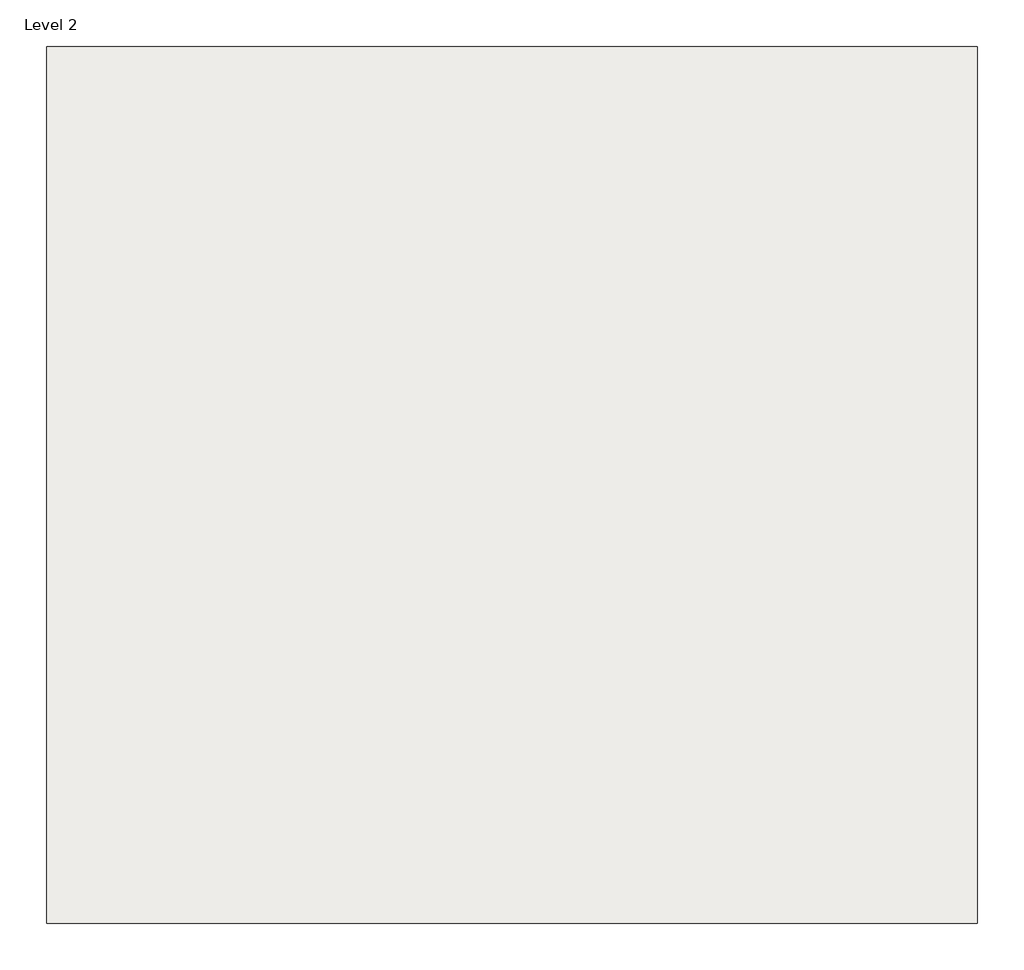
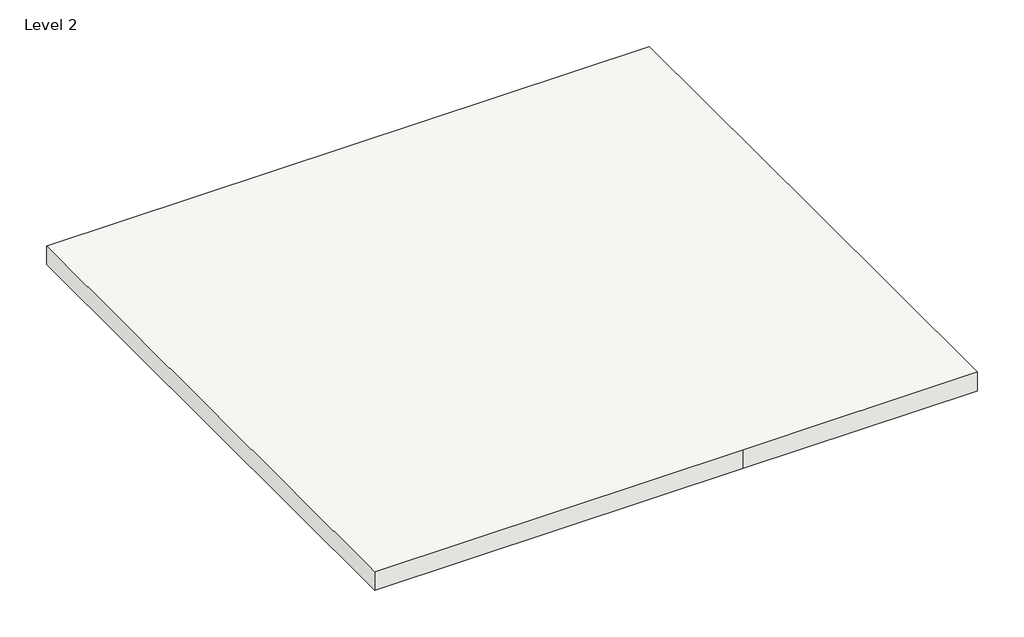
# One storey: 1 roof.
"""IFC4 building model written with IfcOpenShell, lengths in millimetres."""

from ifc_helpers import new_model, si_unit, frame, origin, place, context, project, spatial, polyline, outline, extrude, element, save

model = new_model("IFC4")

# Units and contexts
model_context = context("Model", 3, world=origin())
ifc_project = project(units=[si_unit("LENGTHUNIT", "METRE", prefix="MILLI")], contexts=[model_context])

# Site, building, storey
site = spatial("IfcSite", under=ifc_project)
building = spatial("IfcBuilding", under=site)
storey = spatial("IfcBuildingStorey", under=building, Name="Level 2", Elevation=3048.0)

# Roof
placement = place(None, origin())
element("IfcRoof", 1, ObjectType="Generic - 12\"", at=placement, inside=storey, context=model_context, shape_type="SweptSolid", body=[
    extrude(outline(polyline([(-13352.2770189, 15181.9523405), (-4081.2770189, 15181.9523405), (-4081.2770189, 10762.3523405), (-4081.2770189, 6444.3523405), (-7688.0770189, 6444.3523405), (-13352.2770189, 6444.3523405), (-13352.2770189, 15181.9523405)])), frame((0.0, 0.0, 3048.0), z_axis=(0.0, 0.0, 1.0), x_axis=(1.0, 0.0, 0.0)), (0.0, 0.0, 1.0), 304.8),
])

save(model, "model.ifc")

# Revit data of these elements
# Type "Generic - 12\""
#   Assembly Code = "B1020"
#   Layers, outside or top first: 1' - 0" "Brick, Soldier Course" (function 1)
# Element 1 (IfcRoof, "Generic - 12\"")
#   built-in parameter 1001705 = 11 (stored number, unit not read)
#   built-in parameter 1001710 = 33615
#   Phase Created = New Construction
#   Materials on its faces: "Brick, Soldier Course"
# Materials
#   "Brick, Soldier Course": class "Masonry", colour RGB 170 98 104, transparency 0, Description = "Common brick soldier coursed", Cost = 0
